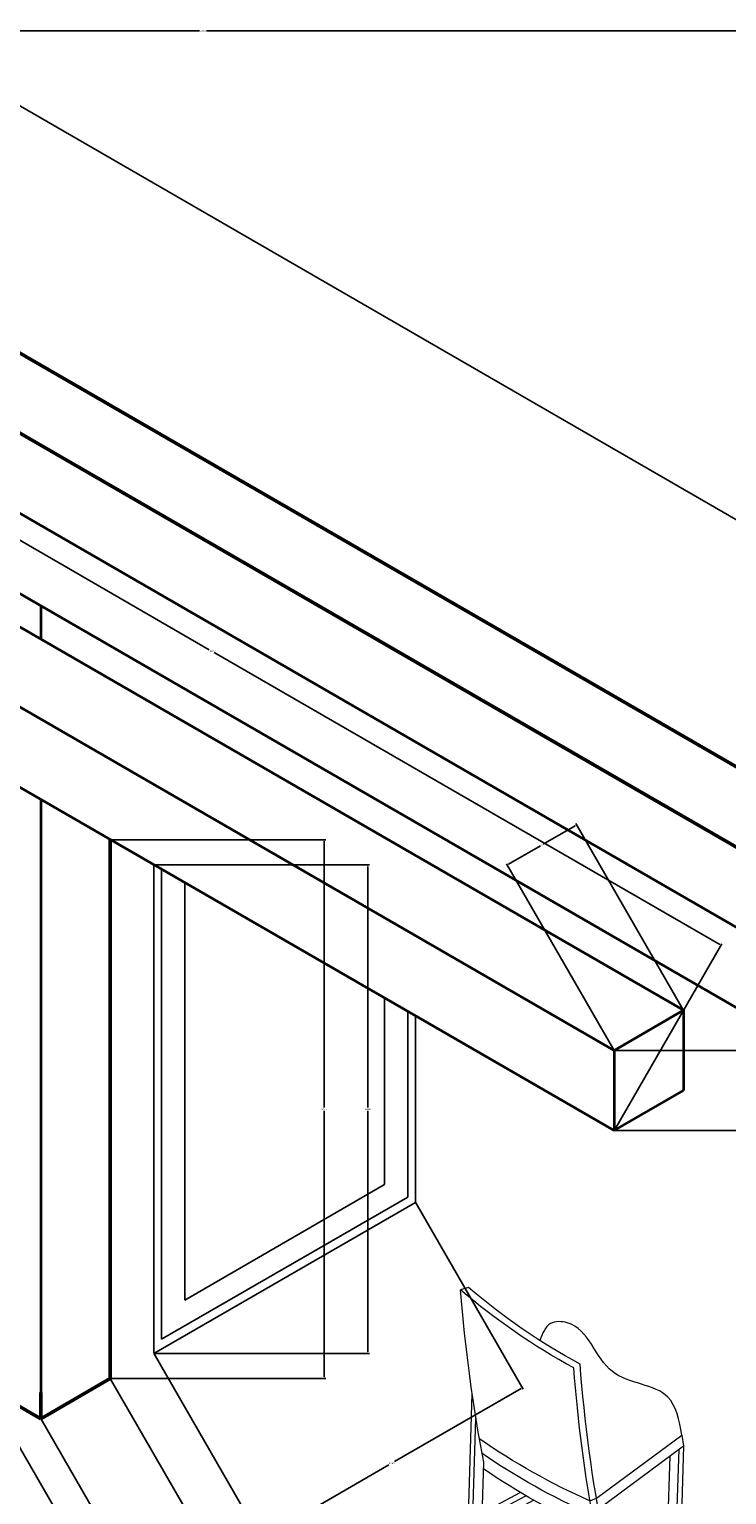
# Model space of a CAD drawing. Units: inches. Extents: x 4150 to 4636, y 2169 to 2592.
# Tile 7 of 8: x 4383 to 4462, y 2428 to 2592. Entities that reach past the tile are written whole.
import ezdxf

# ---------------------------------------------------------------- set-up
doc = ezdxf.new("R2010")
doc.units = ezdxf.units.IN
for name, color, linetype, lineweight in [('A-ANNO-DIMS', 2, 'Continuous', 18), ('A-COLS', 1, 'Continuous', 35), ('A-DOOR', 4, 'Continuous', 25), ('A-FURN', 8, 'Continuous', 18), ('A-WALL', 7, 'Continuous', 50), ('S-BEAM', 1, 'Continuous', 35)]:
    doc.layers.add(name, color=color, linetype=linetype, lineweight=lineweight)
doc.styles.get("Standard").update_dxf_attribs({"font": 'arial.ttf'})
doc.dimstyles.get("Standard").update_dxf_attribs({"dimtxt": 0.18, "dimasz": 0.18, "dimexe": 0.18, "dimexo": 0.0625, "dimgap": 0.09, "dimtad": 0, "dimtih": 1, "dimtoh": 1, "dimdec": 4, "dimzin": 0, "dimdsep": 46, "dimtxsty": 'Standard', "dimcen": 0.09, "dimadec": 0, "dimazin": 0, "dimtfac": 1, "dimtdec": 4, "dimtofl": 0, "dimtmove": 0, "dimatfit": 3, "dimfxl": 1, "dimtolj": 1, "dimtzin": 0, "dimarcsym": 0})

# ---------------------------------------------------------------- blocks, each defined once
blk = doc.blocks.new('CHAIR')
for p, q in [((4460.61, 2323.17), (4462.07, 2322.64)), ((4459.26, 2268.31), (4459.26, 2302.96)), ((4458.4, 2267.81), (4458.4, 2298.32)), ((4419.13, 2296.33), (4418.72, 2294.28)), ((4435.02, 2283.82), (4419.13, 2296.33)), ((4434.61, 2281.77), (4418.72, 2294.28)), ((4418.72, 2294.28), (4418.72, 2263.74)), ((4419.58, 2264.24), (4419.58, 2293.6)), ((4421.31, 2292.24), (4421.31, 2265.24)), ((4456.67, 2268.81), (4456.67, 2290.03)), ((4456.67, 2280.34), (4449.53, 2284.46)), ((4421.31, 2274.06), (4434.6, 2281.73)), ((4436.24, 2283.27), (4435.02, 2283.82)), ((4436.06, 2254.73), (4436.06, 2282.33)), ((4456.67, 2277.45), (4446.94, 2283.07)), ((4456.67, 2279.13), (4448.46, 2283.88)), ((4421.31, 2272.85), (4434.31, 2280.36)), ((4421.31, 2271.17), (4433.9, 2278.43)), ((4433.46, 2255.23), (4433.46, 2276.44)), ((4435.2, 2254.23), (4435.2, 2278.19)), ((4436.06, 2265.55), (4456.67, 2277.45)), ((4436.06, 2264.34), (4456.67, 2276.24)), ((4433.46, 2267.05), (4421.31, 2274.06)), ((4433.46, 2265.84), (4421.31, 2272.85)), ((4436.06, 2262.66), (4456.67, 2274.56)), ((4433.46, 2264.15), (4421.31, 2271.17)), ((4458.4, 2267.81), (4456.67, 2268.81)), ((4458.4, 2267.81), (4459.26, 2268.31)), ((4419.58, 2264.24), (4421.31, 2265.24)), ((4418.72, 2263.74), (4419.58, 2264.24)), ((4435.2, 2254.23), (4433.46, 2255.23)), ((4435.2, 2254.23), (4436.06, 2254.73))]:
    blk.add_line(p, q)
for centre, radius, start, end in [((4387.22, 2413.69), 116.53, 296.3285, 309.0347), ((4384.96, 2418.26), 122.84, 296.6652, 308.8825), ((4169.51, 2354.34), 294.27, 347.3763, 353.8153), ((4146.35, 2340.95), 294.27, 347.3385, 353.8153), ((4147.53, 2340.19), 294.27, 347.8382, 353.8153), ((4388.03, 2401.62), 127.8, 292.164, 302.9931), ((4388.03, 2399.21), 127.8, 292.0735, 302.6755), ((4387.7, 2396.31), 127.8, 292.2346, 302.6625)]:
    blk.add_arc(centre, radius, start, end)
blk.add_open_spline([(4419.13, 2296.33), (4419.73, 2299.09), (4421.22, 2306.03), (4435.02, 2305.47), (4437.67, 2317.36), (4445.4, 2317.24), (4446.24, 2314.8), (4446.7, 2313.47)], degree=3, knots=[0, 0, 0, 0, 7.695976, 19.302291, 31.993754, 35.157842, 38.967805, 38.967805, 38.967805, 38.967805])
blk = doc.blocks.new('*D36')
at = {"layer": 'A-ANNO-DIMS', "color": 0, "lineweight": -2, "transparency": 16777216}
for p, q in [((4174.28, 2460.03), (4174.28, 2592.15)), ((4174.46, 2591.97), (4402.51, 2591.97)), ((4631.36, 2591.97), (4403.31, 2591.97)), ((4631.54, 2412.03), (4631.54, 2592.15))]:
    blk.add_line(p, q, dxfattribs=at)
at = {"layer": 'A-ANNO-DIMS', "color": 0, "transparency": 16777216}
for points in [[(4174.46, 2592), (4174.46, 2591.94), (4174.28, 2591.97)], [(4631.36, 2592), (4631.36, 2591.94), (4631.54, 2591.97)]]:
    blk.add_solid(points, dxfattribs=at)
at = {"layer": 'Defpoints', "color": 0, "transparency": 16777216}
for p in [(4631.54, 2591.97), (4174.28, 2459.97), (4631.54, 2411.97)]:
    blk.add_point(p, dxfattribs=at)
at = {"layer": 'A-ANNO-DIMS', "color": 0, "transparency": 16777216, "insert": (4402.91, 2591.97), "char_height": 0.18, "attachment_point": 5}
blk.add_mtext('\\A1;457.3', dxfattribs=at)
blk = doc.blocks.new('*D37')
at = {"layer": 'A-ANNO-DIMS', "color": 0, "lineweight": -2, "transparency": 16777216}
for p, q in [((4361.28, 2567.97), (4150.1, 2567.97)), ((4150.28, 2567.79), (4150.28, 2379.06)), ((4150.28, 2189.96), (4150.28, 2378.69)), ((4434.34, 2189.78), (4150.1, 2189.78))]:
    blk.add_line(p, q, dxfattribs=at)
at = {"layer": 'A-ANNO-DIMS', "color": 0, "transparency": 16777216}
for points in [[(4150.25, 2567.79), (4150.31, 2567.79), (4150.28, 2567.97)], [(4150.25, 2189.96), (4150.31, 2189.96), (4150.28, 2189.78)]]:
    blk.add_solid(points, dxfattribs=at)
at = {"layer": 'Defpoints', "color": 0, "transparency": 16777216}
for p in [(4361.34, 2567.97), (4150.28, 2189.78), (4434.4, 2189.78)]:
    blk.add_point(p, dxfattribs=at)
at = {"layer": 'A-ANNO-DIMS', "color": 0, "transparency": 16777216, "insert": (4150.28, 2378.87), "char_height": 0.18, "attachment_point": 5}
blk.add_mtext('\\A1;378.2', dxfattribs=at)
blk = doc.blocks.new('*D43')
at = {"layer": 'A-ANNO-DIMS', "color": 0, "lineweight": -2, "transparency": 16777216}
for p, q in [((4361.37, 2568.02), (4373.43, 2588.91)), ((4373.5, 2588.66), (4504.26, 2513.17)), ((4635.59, 2437.34), (4504.83, 2512.83)), ((4623.78, 2416.52), (4635.84, 2437.41))]:
    blk.add_line(p, q, dxfattribs=at)
at = {"layer": 'A-ANNO-DIMS', "color": 0, "transparency": 16777216}
for points in [[(4373.51, 2588.69), (4373.48, 2588.63), (4373.34, 2588.75)], [(4635.61, 2437.37), (4635.58, 2437.31), (4635.75, 2437.25)]]:
    blk.add_solid(points, dxfattribs=at)
at = {"layer": 'Defpoints', "color": 0, "transparency": 16777216}
for p in [(4361.34, 2567.97), (4635.75, 2437.25), (4623.75, 2416.47)]:
    blk.add_point(p, dxfattribs=at)
at = {"layer": 'A-ANNO-DIMS', "color": 0, "transparency": 16777216, "insert": (4504.54, 2513), "char_height": 0.18, "attachment_point": 5}
blk.add_mtext('\\A1;303', dxfattribs=at)
blk = doc.blocks.new('*D45')
at = {"layer": 'A-ANNO-DIMS', "color": 0, "lineweight": -2, "transparency": 16777216}
for p, q in [((4334.77, 2534.66), (4346.83, 2555.54)), ((4346.89, 2555.3), (4403.61, 2522.55)), ((4460.9, 2489.48), (4404.17, 2522.23)), ((4449.08, 2468.66), (4461.14, 2489.54))]:
    blk.add_line(p, q, dxfattribs=at)
at = {"layer": 'A-ANNO-DIMS', "color": 0, "transparency": 16777216}
for points in [[(4346.91, 2555.32), (4346.88, 2555.27), (4346.74, 2555.39)], [(4460.91, 2489.5), (4460.88, 2489.45), (4461.05, 2489.39)]]:
    blk.add_solid(points, dxfattribs=at)
at = {"layer": 'Defpoints', "color": 0, "transparency": 16777216}
for p in [(4334.74, 2534.6), (4461.05, 2489.39), (4449.05, 2468.6)]:
    blk.add_point(p, dxfattribs=at)
at = {"layer": 'A-ANNO-DIMS', "color": 0, "transparency": 16777216, "insert": (4403.89, 2522.39), "char_height": 0.18, "attachment_point": 5}
blk.add_mtext('\\A1;132', dxfattribs=at)
blk = doc.blocks.new('*D46')
at = {"layer": 'A-ANNO-DIMS', "color": 0, "lineweight": -2, "transparency": 16777216}
for p, q in [((4449.11, 2477.6), (4473.23, 2477.6)), ((4473.05, 2477.42), (4473.05, 2473.29)), ((4473.05, 2468.78), (4473.05, 2472.92)), ((4449.11, 2468.6), (4473.23, 2468.6))]:
    blk.add_line(p, q, dxfattribs=at)
at = {"layer": 'A-ANNO-DIMS', "color": 0, "transparency": 16777216}
for points in [[(4473.02, 2477.42), (4473.08, 2477.42), (4473.05, 2477.6)], [(4473.02, 2468.78), (4473.08, 2468.78), (4473.05, 2468.6)]]:
    blk.add_solid(points, dxfattribs=at)
at = {"layer": 'Defpoints', "color": 0, "transparency": 16777216}
for p in [(4449.05, 2477.6), (4449.05, 2468.6), (4473.05, 2468.6)]:
    blk.add_point(p, dxfattribs=at)
at = {"layer": 'A-ANNO-DIMS', "color": 0, "transparency": 16777216, "insert": (4473.05, 2473.1), "char_height": 0.18, "attachment_point": 5}
blk.add_mtext('\\A1;9', dxfattribs=at)
blk = doc.blocks.new('*D47')
at = {"layer": 'A-ANNO-DIMS', "color": 0, "lineweight": -2, "transparency": 16777216}
for p, q in [((4444.69, 2502.8), (4441.1, 2500.73)), ((4456.81, 2482.16), (4444.76, 2503.04)), ((4437.21, 2498.48), (4440.8, 2500.55)), ((4449.02, 2477.66), (4436.96, 2498.54))]:
    blk.add_line(p, q, dxfattribs=at)
at = {"layer": 'A-ANNO-DIMS', "color": 0, "transparency": 16777216}
for points in [[(4444.67, 2502.82), (4444.7, 2502.77), (4444.85, 2502.89)], [(4437.19, 2498.5), (4437.22, 2498.45), (4437.05, 2498.39)]]:
    blk.add_solid(points, dxfattribs=at)
at = {"layer": 'Defpoints', "color": 0, "transparency": 16777216}
for p in [(4444.85, 2502.89), (4456.85, 2482.1), (4449.05, 2477.6)]:
    blk.add_point(p, dxfattribs=at)
at = {"layer": 'A-ANNO-DIMS', "color": 0, "transparency": 16777216, "insert": (4440.95, 2500.64), "char_height": 0.18, "attachment_point": 5}
blk.add_mtext('\\A1;9', dxfattribs=at)
blk = doc.blocks.new('*D49')
at = {"layer": 'A-ANNO-DIMS', "color": 0, "lineweight": -2, "transparency": 16777216}
for p, q in [((4392.55, 2440.74), (4404.61, 2419.85)), ((4384.76, 2436.24), (4396.81, 2415.35)), ((4404.36, 2419.92), (4400.77, 2417.84)), ((4396.88, 2415.6), (4400.47, 2417.67))]:
    blk.add_line(p, q, dxfattribs=at)
at = {"layer": 'A-ANNO-DIMS', "color": 0, "transparency": 16777216}
for points in [[(4404.35, 2419.94), (4404.38, 2419.89), (4404.52, 2420.01)], [(4396.87, 2415.62), (4396.9, 2415.57), (4396.72, 2415.51)]]:
    blk.add_solid(points, dxfattribs=at)
at = {"layer": 'Defpoints', "color": 0, "transparency": 16777216}
for p in [(4392.52, 2440.79), (4384.72, 2436.29), (4396.72, 2415.51)]:
    blk.add_point(p, dxfattribs=at)
at = {"layer": 'A-ANNO-DIMS', "color": 0, "transparency": 16777216, "insert": (4400.62, 2417.76), "char_height": 0.18, "attachment_point": 5}
blk.add_mtext('\\A1;9', dxfattribs=at)
blk = doc.blocks.new('*D50')
at = {"layer": 'A-ANNO-DIMS', "color": 0, "lineweight": -2, "transparency": 16777216}
for p, q in [((4392.58, 2501.24), (4416.7, 2501.24)), ((4416.52, 2501.06), (4416.52, 2471.2)), ((4416.52, 2440.97), (4416.52, 2470.84)), ((4392.58, 2440.79), (4416.7, 2440.79))]:
    blk.add_line(p, q, dxfattribs=at)
at = {"layer": 'A-ANNO-DIMS', "color": 0, "transparency": 16777216}
for points in [[(4416.49, 2501.06), (4416.55, 2501.06), (4416.52, 2501.24)], [(4416.49, 2440.97), (4416.55, 2440.97), (4416.52, 2440.79)]]:
    blk.add_solid(points, dxfattribs=at)
at = {"layer": 'Defpoints', "color": 0, "transparency": 16777216}
for p in [(4392.52, 2501.24), (4392.52, 2440.79), (4416.52, 2440.79)]:
    blk.add_point(p, dxfattribs=at)
at = {"layer": 'A-ANNO-DIMS', "color": 0, "transparency": 16777216, "insert": (4416.52, 2471.02), "char_height": 0.18, "attachment_point": 5}
blk.add_mtext('\\A1;60.45', dxfattribs=at)
blk = doc.blocks.new('*D51')
at = {"layer": 'A-ANNO-DIMS', "color": 0, "lineweight": -2, "transparency": 16777216}
for p, q in [((4426.8, 2460.49), (4438.85, 2439.61)), ((4397.44, 2443.55), (4409.5, 2422.66)), ((4438.61, 2439.67), (4424.4, 2431.47)), ((4409.57, 2422.91), (4423.77, 2431.11))]:
    blk.add_line(p, q, dxfattribs=at)
at = {"layer": 'A-ANNO-DIMS', "color": 0, "transparency": 16777216}
for points in [[(4438.59, 2439.7), (4438.62, 2439.65), (4438.76, 2439.76)], [(4409.55, 2422.93), (4409.58, 2422.88), (4409.41, 2422.82)]]:
    blk.add_solid(points, dxfattribs=at)
at = {"layer": 'Defpoints', "color": 0, "transparency": 16777216}
for p in [(4426.76, 2460.55), (4397.41, 2443.6), (4409.41, 2422.82)]:
    blk.add_point(p, dxfattribs=at)
at = {"layer": 'A-ANNO-DIMS', "color": 0, "transparency": 16777216, "insert": (4424.09, 2431.29), "char_height": 0.18, "attachment_point": 5}
blk.add_mtext('\\A1;33.89', dxfattribs=at)
blk = doc.blocks.new('*D52')
at = {"layer": 'A-ANNO-DIMS', "color": 0, "lineweight": -2, "transparency": 16777216}
for p, q in [((4397.47, 2498.42), (4421.59, 2498.42)), ((4421.41, 2498.24), (4421.41, 2471.19)), ((4421.41, 2443.78), (4421.41, 2470.83)), ((4397.47, 2443.6), (4421.59, 2443.6))]:
    blk.add_line(p, q, dxfattribs=at)
at = {"layer": 'A-ANNO-DIMS', "color": 0, "transparency": 16777216}
for points in [[(4421.38, 2498.24), (4421.44, 2498.24), (4421.41, 2498.42)], [(4421.38, 2443.78), (4421.44, 2443.78), (4421.41, 2443.6)]]:
    blk.add_solid(points, dxfattribs=at)
at = {"layer": 'Defpoints', "color": 0, "transparency": 16777216}
for p in [(4397.41, 2498.42), (4397.41, 2443.6), (4421.41, 2443.6)]:
    blk.add_point(p, dxfattribs=at)
at = {"layer": 'A-ANNO-DIMS', "color": 0, "transparency": 16777216, "insert": (4421.41, 2471.01), "char_height": 0.18, "attachment_point": 5}
blk.add_mtext('\\A1;54.82', dxfattribs=at)
blk = doc.blocks.new('*D55')
at = {"layer": 'A-ANNO-DIMS', "color": 0, "lineweight": -2, "transparency": 16777216}
for p, q in [((4380.31, 2436.61), (4392.37, 2415.73)), ((4392.12, 2415.79), (4308.21, 2367.35)), ((4223.67, 2318.54), (4307.58, 2366.99)), ((4211.55, 2339.18), (4223.61, 2318.3))]:
    blk.add_line(p, q, dxfattribs=at)
at = {"layer": 'A-ANNO-DIMS', "color": 0, "transparency": 16777216}
for points in [[(4392.11, 2415.82), (4392.14, 2415.77), (4392.28, 2415.88)], [(4223.66, 2318.57), (4223.69, 2318.52), (4223.52, 2318.45)]]:
    blk.add_solid(points, dxfattribs=at)
at = {"layer": 'Defpoints', "color": 0, "transparency": 16777216}
for p in [(4380.28, 2436.67), (4211.52, 2339.24), (4223.52, 2318.45)]:
    blk.add_point(p, dxfattribs=at)
at = {"layer": 'A-ANNO-DIMS', "color": 0, "transparency": 16777216, "insert": (4307.9, 2367.17), "char_height": 0.18, "attachment_point": 5}
blk.add_mtext('\\A1;194.86', dxfattribs=at)

msp = doc.modelspace()

# ---------------------------------------------------------------- linework, layer by layer
at = {"layer": 'A-COLS'}
msp.add_line((4384.7242, 2505.7435), (4384.7242, 2438.3497), dxfattribs=at)
at = {"layer": 'A-DOOR'}
for p, q in [((4397.4119, 2498.4182), (4397.4119, 2443.6015)), ((4398.278, 2497.9182), (4398.278, 2445.2004)), ((4400.876, 2496.4182), (4400.876, 2449.6015)), ((4423.3001, 2462.548), (4423.3001, 2483.4716)), ((4425.8982, 2461.1469), (4425.8982, 2481.9716)), ((4426.7642, 2460.548), (4426.7642, 2481.4716)), ((4400.876, 2449.6015), (4423.3001, 2462.548)), ((4398.278, 2445.2004), (4425.8982, 2461.1469)), ((4397.4119, 2443.6015), (4426.7642, 2460.548))]:
    msp.add_line(p, q, dxfattribs=at)
at = {"layer": 'A-WALL'}
for p, q in [((4361.3415, 2567.9652), (4506.8337, 2483.9652)), ((4361.3415, 2558.9652), (4615.9529, 2411.9652)), ((4361.3415, 2558.9652), (4454.8722, 2504.9652)), ((4392.5184, 2440.7926), (4392.5184, 2501.2435)), ((4384.7242, 2436.2926), (4392.5184, 2440.7926)), ((4384.7242, 2436.2926), (4380.3446, 2438.8212)), ((4384.7242, 2439.2364), (4384.7242, 2436.2926))]:
    msp.add_line(p, q, dxfattribs=at)
at = {"layer": 'S-BEAM'}
for p, q in [((4353.5472, 2554.4652), (4467.8626, 2488.4652)), ((4342.5299, 2548.1043), (4456.8453, 2482.1043)), ((4353.5472, 2545.4652), (4466.3233, 2480.3539)), ((4334.7357, 2543.6043), (4449.0511, 2477.6043)), ((4334.7357, 2534.6043), (4449.0511, 2468.6043)), ((4384.7242, 2527.4652), (4384.7242, 2523.7435)), ((4456.8453, 2482.1043), (4449.0511, 2477.6043)), ((4456.8453, 2482.1043), (4456.8453, 2473.1043)), ((4449.0511, 2477.6043), (4449.0511, 2468.6043)), ((4449.0511, 2468.6043), (4456.8453, 2473.1043))]:
    msp.add_line(p, q, dxfattribs=at)

# ---------------------------------------------------------------- block references
at = {"layer": 'A-FURN', "xscale": -0.589443472789305, "yscale": 0.589443472789305, "zscale": 0.5894434727893052, "rotation": 358.2313469525009}
msp.add_blockref('CHAIR', (7018.4597, 1001.1473), dxfattribs=at)

# ---------------------------------------------------------------- dimensions: what is measured, and where the dimension line sits
at = {"layer": 'A-ANNO-DIMS'}
dim = msp.add_linear_dim(base=(4631.5414, 2591.9652), p1=(4174.28, 2459.9652), p2=(4631.5414, 2411.9652), dimstyle='Standard', override={"dimdec": 1, "dimlfac": 1, "dimrnd": 0, "dimzin": 0, "dimdsep": 46, "dimlunit": 2}, dxfattribs=at)
dim.commit()
dim.dimension.update_dxf_attribs({"geometry": '*D36', "text_midpoint": (4402.9107, 2591.9652)})
for base, p1, p2, angle, override, picture, middle in [((4635.7472, 2437.2498), (4361.3415, 2567.9652), (4623.7472, 2416.4652), 330, {"dimdec": 0, "dimlfac": 1, "dimrnd": 0, "dimzin": 0, "dimdsep": 46, "dimlunit": 2}, '*D43', (4504.5443, 2512.9998)), ((4150.28, 2189.7836), (4361.3415, 2567.9652), (4434.4021, 2189.7836), 90, {"dimdec": 1, "dimlfac": 1, "dimrnd": 0, "dimzin": 0, "dimdsep": 46, "dimlunit": 2}, '*D37', (4150.28, 2378.8744)), ((4461.0511, 2489.3889), (4334.7357, 2534.6043), (4449.0511, 2468.6043), 330, {"dimdec": 0, "dimlfac": 1, "dimrnd": 0, "dimzin": 0, "dimdsep": 46, "dimlunit": 2}, '*D45', (4403.8934, 2522.3889)), ((4444.8453, 2502.8889), (4449.0511, 2477.6043), (4456.8453, 2482.1043), 30, {"dimdec": 0, "dimlfac": 1, "dimrnd": 0, "dimzin": 0, "dimdsep": 46, "dimlunit": 2}, '*D47', (4440.9482, 2500.6389)), ((4416.5184, 2440.7926), (4392.5184, 2501.2435), (4392.5184, 2440.7926), 270, {"dimdec": 2, "dimlfac": 1, "dimrnd": 0, "dimzin": 0, "dimdsep": 46, "dimlunit": 2}, '*D50', (4416.5184, 2471.0181)), ((4421.4119, 2443.6015), (4397.4119, 2498.4182), (4397.4119, 2443.6015), 270, {"dimdec": 2, "dimlfac": 1, "dimrnd": 0, "dimzin": 0, "dimdsep": 46, "dimlunit": 2}, '*D52', (4421.4119, 2471.0098)), ((4473.0511, 2468.6043), (4449.0511, 2477.6043), (4449.0511, 2468.6043), 270, {"dimdec": 0, "dimlfac": 1, "dimrnd": 0, "dimzin": 0, "dimdsep": 46, "dimlunit": 2}, '*D46', (4473.0511, 2473.1043)), ((4409.4119, 2422.8168), (4426.7642, 2460.548), (4397.4119, 2443.6015), 210, {"dimdec": 2, "dimlfac": 1, "dimrnd": 0, "dimzin": 0, "dimdsep": 46, "dimlunit": 2}, '*D51', (4424.0881, 2431.2901)), ((4396.7242, 2415.508), (4392.5184, 2440.7926), (4384.7242, 2436.2926), 210, {"dimdec": 0, "dimlfac": 1, "dimrnd": 0, "dimzin": 0, "dimdsep": 46, "dimlunit": 2}, '*D49', (4400.6213, 2417.758)), ((4223.5191, 2318.4518), (4380.2767, 2436.6687), (4211.5191, 2339.2364), 210, {"dimdec": 2, "dimlfac": 1, "dimrnd": 0, "dimzin": 0, "dimdsep": 46, "dimlunit": 2}, '*D55', (4307.8979, 2367.1679))]:
    dim = msp.add_linear_dim(base=base, p1=p1, p2=p2, angle=angle, dimstyle='Standard', override=override, dxfattribs=at)
    dim.commit()
    dim.dimension.update_dxf_attribs({"geometry": picture, "text_midpoint": middle})

doc.saveas('drawing.dxf')
